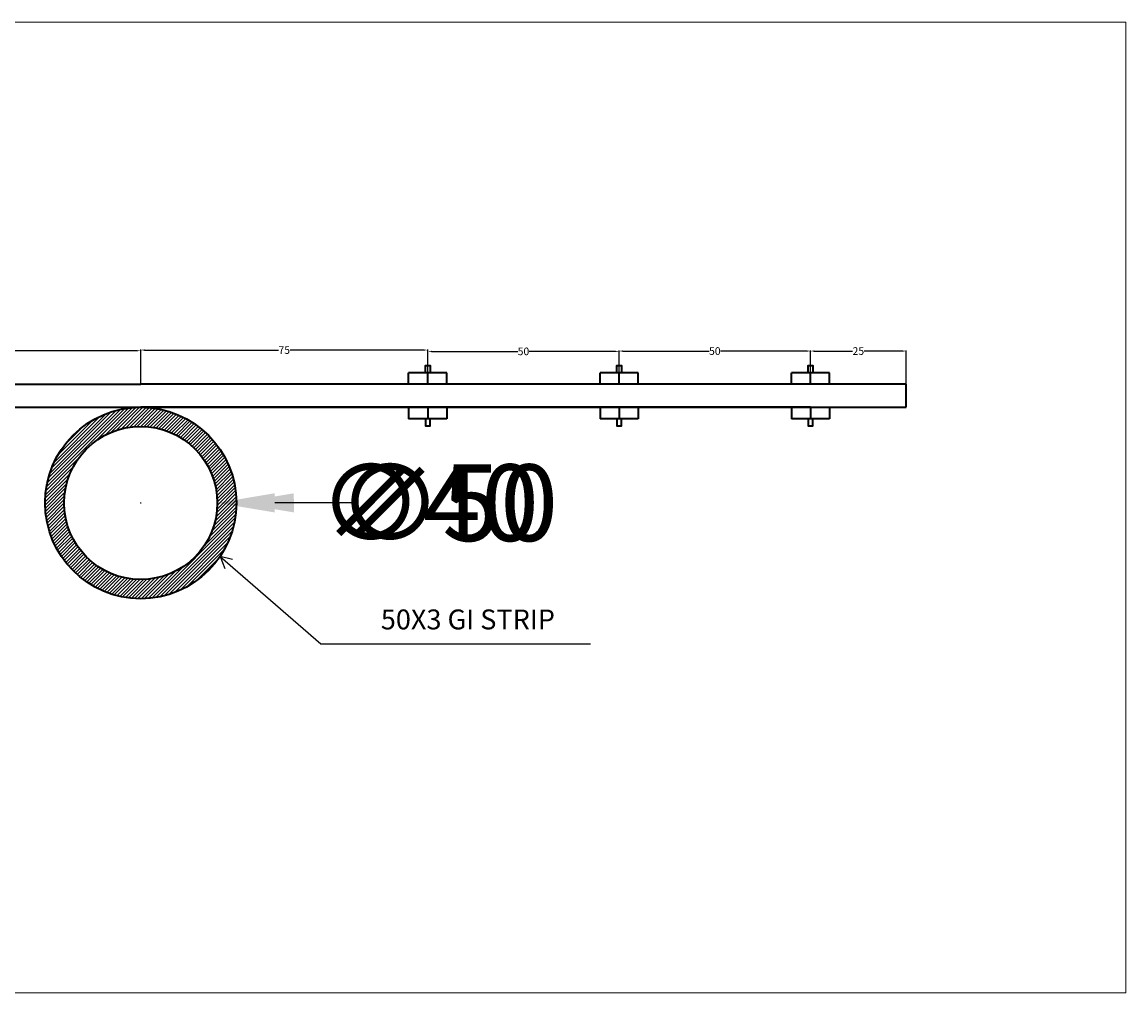
# Model space of a CAD drawing. Units: inches. Extents: x -129 to 2013, y -3652 to 814.
# Tile 3 of 5: x 387 to 675, y -1618 to -1364. Entities that reach past the tile are written whole.
import ezdxf

# ---------------------------------------------------------------- set-up
doc = ezdxf.new("R2010")
doc.units = ezdxf.units.IN
doc.header["$MEASUREMENT"] = 0
for name, color, linetype, lineweight in [('A-ANNO-DIMS', 2, 'Continuous', 18), ('A-ANNO-SYMB', 3, 'Continuous', 18), ('A-ANNO-TEXT', 7, 'Continuous', 25), ('A-DETL-PATT', 8, 'Continuous', 13), ('E-GRND', 1, 'Continuous', 35)]:
    doc.layers.add(name, color=color, linetype=linetype, lineweight=lineweight)
doc.styles.get("Standard").update_dxf_attribs({"font": 'arial.ttf'})
doc.dimstyles.new('SMALL', dxfattribs={"dimtxt": 2, "dimasz": 1, "dimexe": 0.18, "dimexo": 0.0625, "dimgap": 0.09, "dimtad": 0, "dimdec": 0, "dimzin": 0, "dimdsep": 46, "dimtxsty": 'Standard', "dimcen": 0.09, "dimadec": 0, "dimazin": 0, "dimtfac": 1, "dimtdec": 0, "dimtofl": 0, "dimtmove": 0, "dimatfit": 3, "dimfxl": 1, "dimtolj": 1, "dimtzin": 0, "dimarcsym": 0})
doc.dimstyles.get("Standard").update_dxf_attribs({"dimtxt": 20, "dimasz": 15, "dimexe": 0.18, "dimexo": 0.0625, "dimgap": 0.09, "dimtad": 0, "dimdec": 0, "dimzin": 0, "dimdsep": 46, "dimtxsty": 'Standard', "dimcen": 0.09, "dimadec": 0, "dimazin": 0, "dimtfac": 1, "dimtdec": 0, "dimtofl": 0, "dimtmove": 0, "dimatfit": 3, "dimfxl": 1, "dimtolj": 1, "dimtzin": 0, "dimarcsym": 0})

# ---------------------------------------------------------------- blocks, each defined once
blk = doc.blocks.new('*D14')
at = {"layer": 'A-ANNO-DIMS', "color": 0, "lineweight": -2, "transparency": 16777216}
for p, q in [((342.51, -1458.55), (342.51, -1449.69)), ((343.51, -1449.87), (378.49, -1449.87)), ((416.51, -1449.87), (381.54, -1449.87)), ((417.51, -1458.55), (417.51, -1449.69))]:
    blk.add_line(p, q, dxfattribs=at)
at = {"layer": 'A-ANNO-DIMS', "color": 0, "transparency": 16777216}
for points in [[(343.51, -1449.7), (343.51, -1450.03), (342.51, -1449.87)], [(416.51, -1449.7), (416.51, -1450.03), (417.51, -1449.87)]]:
    blk.add_solid(points, dxfattribs=at)
at = {"layer": 'Defpoints', "color": 0, "transparency": 16777216}
for p in [(417.51, -1449.87), (342.51, -1458.61), (417.51, -1458.61)]:
    blk.add_point(p, dxfattribs=at)
at = {"layer": 'A-ANNO-DIMS', "color": 0, "transparency": 16777216, "insert": (380.01, -1449.87), "char_height": 2, "attachment_point": 5}
blk.add_mtext('\\A1;75', dxfattribs=at)
blk = doc.blocks.new('*D15')
at = {"layer": 'A-ANNO-DIMS', "color": 0, "lineweight": -2, "transparency": 16777216}
for p, q in [((492.51, -1458.55), (492.51, -1449.85)), ((493.51, -1450.03), (516, -1450.03)), ((541.51, -1450.03), (519.03, -1450.03)), ((542.51, -1458.55), (542.51, -1449.85))]:
    blk.add_line(p, q, dxfattribs=at)
at = {"layer": 'A-ANNO-DIMS', "color": 0, "transparency": 16777216}
for points in [[(493.51, -1449.87), (493.51, -1450.2), (492.51, -1450.03)], [(541.51, -1449.87), (541.51, -1450.2), (542.51, -1450.03)]]:
    blk.add_solid(points, dxfattribs=at)
at = {"layer": 'Defpoints', "color": 0, "transparency": 16777216}
for p in [(542.51, -1450.03), (492.51, -1458.61), (542.51, -1458.61)]:
    blk.add_point(p, dxfattribs=at)
at = {"layer": 'A-ANNO-DIMS', "color": 0, "transparency": 16777216, "insert": (517.51, -1450.03), "char_height": 2, "attachment_point": 5}
blk.add_mtext('\\A1;50', dxfattribs=at)
blk = doc.blocks.new('*D16')
at = {"layer": 'A-ANNO-DIMS', "color": 0, "lineweight": -2, "transparency": 16777216}
for p, q in [((542.51, -1458.55), (542.51, -1449.77)), ((543.51, -1449.95), (566, -1449.95)), ((591.51, -1449.95), (569.03, -1449.95)), ((592.51, -1458.55), (592.51, -1449.77))]:
    blk.add_line(p, q, dxfattribs=at)
at = {"layer": 'A-ANNO-DIMS', "color": 0, "transparency": 16777216}
for points in [[(543.51, -1449.78), (543.51, -1450.12), (542.51, -1449.95)], [(591.51, -1449.78), (591.51, -1450.12), (592.51, -1449.95)]]:
    blk.add_solid(points, dxfattribs=at)
at = {"layer": 'Defpoints', "color": 0, "transparency": 16777216}
for p in [(542.51, -1449.95), (542.51, -1458.61), (592.51, -1458.61)]:
    blk.add_point(p, dxfattribs=at)
at = {"layer": 'A-ANNO-DIMS', "color": 0, "transparency": 16777216, "insert": (567.51, -1449.95), "char_height": 2, "attachment_point": 5}
blk.add_mtext('\\A1;50', dxfattribs=at)
blk = doc.blocks.new('*D17')
at = {"layer": 'A-ANNO-DIMS', "color": 0, "lineweight": -2, "transparency": 16777216}
for p, q in [((592.51, -1458.55), (592.51, -1449.77)), ((593.51, -1449.95), (603.47, -1449.95)), ((616.51, -1449.95), (606.56, -1449.95)), ((617.51, -1458.55), (617.51, -1449.77))]:
    blk.add_line(p, q, dxfattribs=at)
at = {"layer": 'A-ANNO-DIMS', "color": 0, "transparency": 16777216}
for points in [[(593.51, -1449.78), (593.51, -1450.12), (592.51, -1449.95)], [(616.51, -1449.78), (616.51, -1450.12), (617.51, -1449.95)]]:
    blk.add_solid(points, dxfattribs=at)
at = {"layer": 'Defpoints', "color": 0, "transparency": 16777216}
for p in [(592.51, -1449.95), (592.51, -1458.61), (617.51, -1458.61)]:
    blk.add_point(p, dxfattribs=at)
at = {"layer": 'A-ANNO-DIMS', "color": 0, "transparency": 16777216, "insert": (605.01, -1449.95), "char_height": 2, "attachment_point": 5}
blk.add_mtext('\\A1;25', dxfattribs=at)
blk = doc.blocks.new('*D18')
at = {"layer": 'A-ANNO-DIMS', "color": 0, "lineweight": -2, "transparency": 16777216}
for p, q in [((417.51, -1458.55), (417.51, -1449.51)), ((418.51, -1449.69), (453.49, -1449.69)), ((491.51, -1449.69), (456.54, -1449.69)), ((492.51, -1458.55), (492.51, -1449.51))]:
    blk.add_line(p, q, dxfattribs=at)
at = {"layer": 'A-ANNO-DIMS', "color": 0, "transparency": 16777216}
for points in [[(418.51, -1449.52), (418.51, -1449.85), (417.51, -1449.69)], [(491.51, -1449.52), (491.51, -1449.85), (492.51, -1449.69)]]:
    blk.add_solid(points, dxfattribs=at)
at = {"layer": 'Defpoints', "color": 0, "transparency": 16777216}
for p in [(492.51, -1449.69), (417.51, -1458.61), (492.51, -1458.61)]:
    blk.add_point(p, dxfattribs=at)
at = {"layer": 'A-ANNO-DIMS', "color": 0, "transparency": 16777216, "insert": (455.01, -1449.69), "char_height": 2, "attachment_point": 5}
blk.add_mtext('\\A1;75', dxfattribs=at)
blk = doc.blocks.new('BOLT-M10-MIR')
for p, q in [((587.51, -1458.61), (587.51, -1455.61)), ((597.51, -1455.61), (587.51, -1455.61)), ((592.51, -1458.61), (592.51, -1455.61)), ((597.51, -1458.61), (597.51, -1455.61)), ((587.51, -1464.61), (587.51, -1467.61)), ((592.51, -1464.61), (592.51, -1467.61)), ((597.51, -1464.61), (597.51, -1467.61)), ((597.51, -1467.61), (587.51, -1467.61))]:
    blk.add_line(p, q)
for points in [[(593.14, -1455.61), (591.89, -1455.61), (591.89, -1453.74), (593.14, -1453.74)], [(593.14, -1467.61), (591.89, -1467.61), (591.89, -1469.49), (593.14, -1469.49)]]:
    blk.add_lwpolyline(points, close=True)
blk = doc.blocks.new('*D35')
at = {"layer": 'A-ANNO-DIMS', "color": 0, "lineweight": -2, "transparency": 16777216}
for p, q in [((417.42, -1489.61), (417.6, -1489.61)), ((417.51, -1489.7), (417.51, -1489.52)), ((472.51, -1489.58), (457.51, -1489.59))]:
    blk.add_line(p, q, dxfattribs=at)
at = {"layer": 'A-ANNO-DIMS', "color": 0, "transparency": 16777216}
blk.add_solid([(457.51, -1487.09), (457.52, -1492.09), (442.51, -1489.6)], dxfattribs=at)
at = {"layer": 'Defpoints', "color": 0, "transparency": 16777216}
for p in [(392.51, -1489.63), (442.51, -1489.6)]:
    blk.add_point(p, dxfattribs=at)
at = {"layer": 'A-ANNO-DIMS', "color": 0, "transparency": 16777216, "insert": (497.78, -1489.57), "char_height": 20, "attachment_point": 5, "rotation": 0.0311}
blk.add_mtext('\\A1;∅50', dxfattribs=at)
blk = doc.blocks.new('*D36')
at = {"layer": 'A-ANNO-DIMS', "color": 0, "lineweight": -2, "transparency": 16777216}
for p, q in [((417.42, -1489.61), (417.6, -1489.61)), ((417.51, -1489.7), (417.51, -1489.52)), ((467.51, -1489.58), (452.51, -1489.59))]:
    blk.add_line(p, q, dxfattribs=at)
at = {"layer": 'A-ANNO-DIMS', "color": 0, "transparency": 16777216}
blk.add_solid([(452.51, -1487.09), (452.52, -1492.09), (437.51, -1489.6)], dxfattribs=at)
at = {"layer": 'Defpoints', "color": 0, "transparency": 16777216}
for p in [(397.51, -1489.63), (437.51, -1489.6)]:
    blk.add_point(p, dxfattribs=at)
at = {"layer": 'A-ANNO-DIMS', "color": 0, "transparency": 16777216, "insert": (492.78, -1489.56), "char_height": 20, "attachment_point": 5, "rotation": 0.0388}
blk.add_mtext('\\A1;∅40', dxfattribs=at)

msp = doc.modelspace()

# ---------------------------------------------------------------- hatches: boundary and pattern name
at = {"layer": 'A-DETL-PATT'}
h = msp.add_hatch(dxfattribs=at)
h.set_pattern_fill('ANSI31', color=256, scale=5)
h.set_pattern_definition([(45, (773.4427, 0), (-0.44194174, 0.44194174), [])])
h.paths.add_polyline_path([(392.5146, -1489.6135, 1), (442.5146, -1489.6135, 1)])
h.paths.add_polyline_path([(437.5146, -1489.6135, -1), (397.5146, -1489.6135, -1)], flags=16)

# ---------------------------------------------------------------- linework, layer by layer
at = {"layer": 'A-ANNO-SYMB'}
msp.add_lwpolyline([(674.9231, -1617.5657), (98.0927, -1617.5657), (98.0927, -1364.0415), (674.9231, -1364.0415)], close=True, dxfattribs=at)
at = {"layer": 'A-ANNO-TEXT'}
for points in [[(438.2269, -1503.6135), (464.6014, -1526.4409), (535.056, -1526.4409)], [(441.4893, -1504.3903), (438.2269, -1503.6135), (439.4614, -1506.7316)]]:
    msp.add_lwpolyline(points, dxfattribs=at)
at = {"layer": 'E-GRND'}
for p, q in [((342.5146, -1458.6135), (417.5146, -1458.6135)), ((492.5146, -1458.6135), (417.5146, -1458.6135)), ((542.5146, -1458.6135), (492.5146, -1458.6135)), ((542.5146, -1458.6135), (492.5146, -1458.6135)), ((592.5146, -1458.6135), (542.5146, -1458.6135)), ((592.5146, -1458.6135), (542.5146, -1458.6135)), ((617.5146, -1458.6135), (592.5146, -1458.6135)), ((617.5146, -1464.6135), (617.5146, -1458.6135)), ((217.5146, -1464.6135), (617.5146, -1464.6135)), ((342.5146, -1464.6135), (417.5146, -1464.6135)), ((492.5146, -1464.6135), (417.5146, -1464.6135)), ((542.5146, -1464.6135), (492.5146, -1464.6135)), ((542.5146, -1464.6135), (492.5146, -1464.6135)), ((592.5146, -1464.6135), (542.5146, -1464.6135)), ((592.5146, -1464.6135), (542.5146, -1464.6135))]:
    msp.add_line(p, q, dxfattribs=at)
for radius in [25, 20]:
    msp.add_circle((417.5146, -1489.6135), radius, dxfattribs=at)

# ---------------------------------------------------------------- block references
for p in [(-100, 0), (-50, 0), (0, 0)]:
    msp.add_blockref('BOLT-M10-MIR', p, dxfattribs=at)

# ---------------------------------------------------------------- texts
at = {"layer": 'A-ANNO-TEXT'}
msp.add_text('50X3 GI STRIP', height=5.191665, dxfattribs=at).set_placement((480.2408, -1522.6321))

# ---------------------------------------------------------------- dimensions: what is measured, and where the dimension line sits
at = {"layer": 'A-ANNO-DIMS'}
for base, p1, p2, picture, middle in [((417.5146, -1449.8672), (342.5146, -1458.6135), (417.5146, -1458.6135), '*D14', (380.0146, -1449.8672)), ((492.5146, -1449.6872), (417.5146, -1458.6135), (492.5146, -1458.6135), '*D18', (455.0146, -1449.6872)), ((542.5146, -1450.0338), (492.5146, -1458.6135), (542.5146, -1458.6135), '*D15', (517.5146, -1450.0338)), ((542.5146, -1449.9505), (592.5146, -1458.6135), (542.5146, -1458.6135), '*D16', (567.5146, -1449.9505)), ((592.5146, -1449.9505), (617.5146, -1458.6135), (592.5146, -1458.6135), '*D17', (605.0146, -1449.9505))]:
    dim = msp.add_linear_dim(base=base, p1=p1, p2=p2, dimstyle='SMALL', override={"dimclrd": 0, "dimclre": 0, "dimclrt": 0}, dxfattribs=at)
    dim.commit()
    dim.dimension.update_dxf_attribs({"geometry": picture, "text_midpoint": middle})
for p1, p2, picture, middle in [((392.5146, -1489.6271), (442.5146, -1489.6), '*D35', (497.7751, -1489.57)), ((397.5146, -1489.6271), (437.5146, -1489.6), '*D36', (492.7751, -1489.5625))]:
    dim = msp.add_diameter_dim_2p(p1=p1, p2=p2, dimstyle='Standard', override={"dimdec": 0, "dimlfac": 1, "dimrnd": 0, "dimzin": 0, "dimdsep": 46, "dimlunit": 2}, dxfattribs=at)
    dim.commit()
    dim.dimension.update_dxf_attribs({"geometry": picture, "text_midpoint": middle, "dimtype": 163})

doc.saveas('drawing.dxf')
